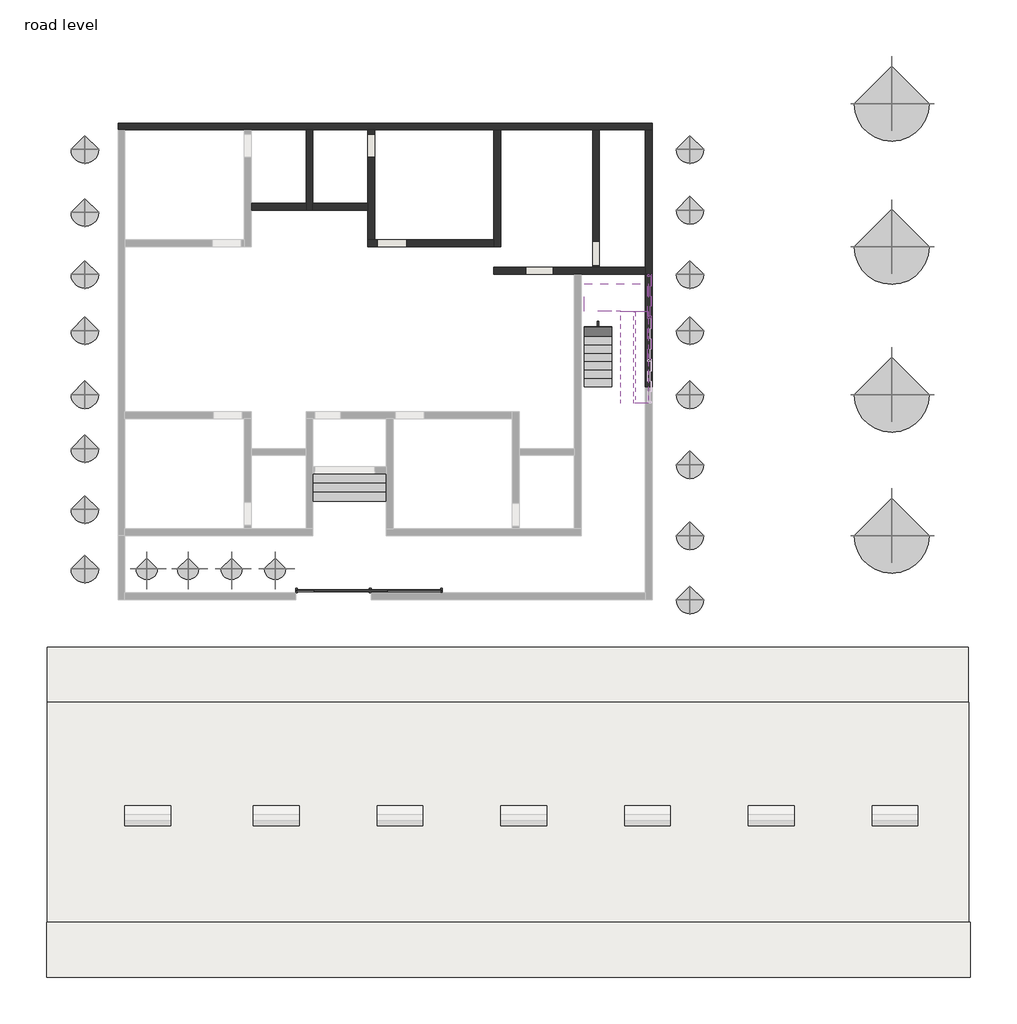
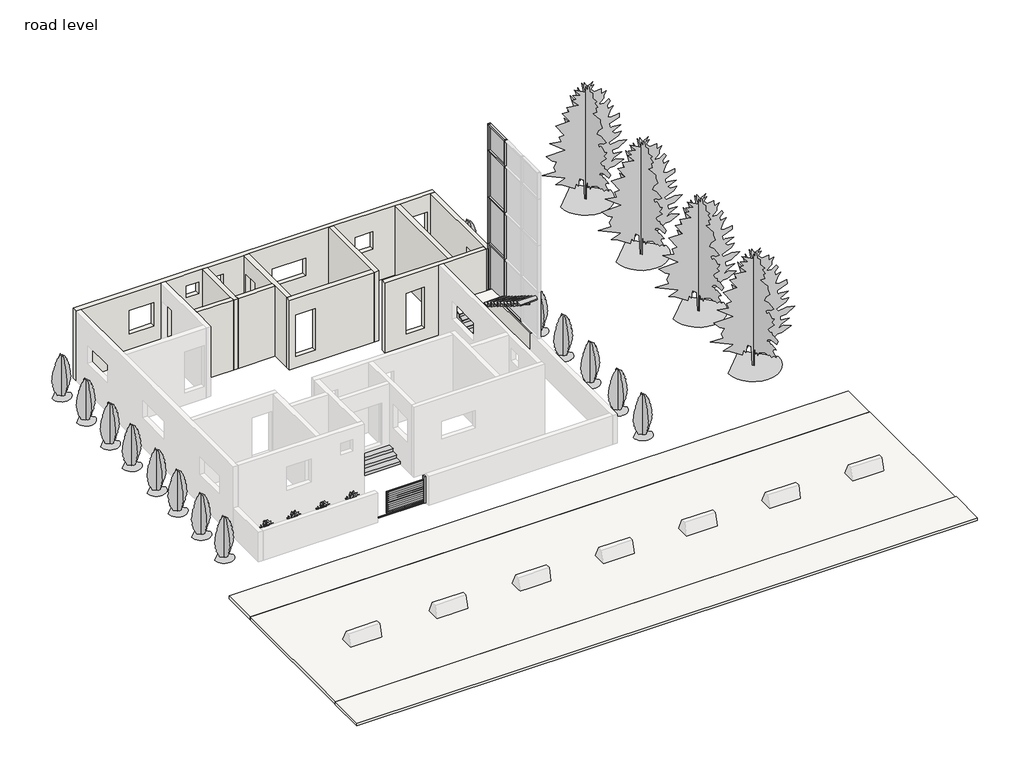
# One storey, part 2 of 2: 25 geographic elements, 16 members, 11 walls, 4 plates, 4 slabs, 2 stair flights, 1 furniture element.
"""IFC4 building model written with IfcOpenShell, lengths in millimetres."""

from ifc_helpers import new_model, si_unit, frame, origin, origin_with_axes, place, context, project, spatial, polyline, outline, extrude, faceted_brep, transform, mapped, element, save
from components import casework_1_casework_1_59e189ff, rpc_plant_tropical_5a024449, rpc_tree_conifer_331a7903, rpc_tree_conifer_chinese_juniper_7_1b9786cd, sliding_gate_17236_sliding_gate_17236_fdb57db6, member_6e705821, member_22948727, member_0bf151aa, member_f0fea5a5, member_ee409385, member_824a4a8d, member_c6627131, system_panel_glazed_532211e4, system_panel_glazed_e2c3efe7, system_panel_glazed_7e5d82eb, non_monolithic_landing_cdb44c8c, stair_flight_ed17b8c2, stair_flight_ca9b9272

model = new_model("IFC4")

# Units and contexts
model_context = context("Model", 3, world=origin())
ifc_project = project(units=[si_unit("LENGTHUNIT", "METRE", prefix="MILLI")], contexts=[model_context])

# Site, building, storey
site = spatial("IfcSite", under=ifc_project)
building = spatial("IfcBuilding", under=site)
storey = spatial("IfcBuildingStorey", under=building, Name="road level", Elevation=0.0)

# Furniture
placement = place(None, origin())
casework_1_casework_1_shape = casework_1_casework_1_59e189ff(model_context)
element("IfcFurniture", 1, ObjectType="Casework 1 : Casework 1", at=placement, inside=storey, context=model_context, shape_type="MappedRepresentation", body=[
    mapped(casework_1_casework_1_shape, transform((0.0, 2082.8, -1435.1), x_axis=(1.0, 0.0, 0.0), y_axis=(0.0, 1.0, 0.0), z_axis=(0.0, 0.0, 1.0))),
])

# Geographic elements
rpc_plant_tropical_shape = rpc_plant_tropical_5a024449(model_context)
element("IfcGeographicElement", 2, ObjectType="RPC Plant - Tropical", at=placement, inside=storey, context=model_context, shape_type="MappedRepresentation", body=[
    mapped(rpc_plant_tropical_shape, transform((-7077.0739162, -7746.9339187, 0.0), x_axis=(1.0, 0.0, 0.0), y_axis=(0.0, 1.0, 0.0), z_axis=(0.0, 0.0, 1.0))),
])
element("IfcGeographicElement", 3, ObjectType="RPC Plant - Tropical", at=placement, inside=storey, context=model_context, shape_type="MappedRepresentation", body=[
    mapped(rpc_plant_tropical_shape, transform((-5705.4739162, -7746.9339187, 0.0), x_axis=(1.0, 0.0, 0.0), y_axis=(0.0, 1.0, 0.0), z_axis=(0.0, 0.0, 1.0))),
])
element("IfcGeographicElement", 4, ObjectType="RPC Plant - Tropical", at=placement, inside=storey, context=model_context, shape_type="MappedRepresentation", body=[
    mapped(rpc_plant_tropical_shape, transform((-4257.6739162, -7746.9339187, 0.0), x_axis=(1.0, 0.0, 0.0), y_axis=(0.0, 1.0, 0.0), z_axis=(0.0, 0.0, 1.0))),
])
element("IfcGeographicElement", 5, ObjectType="RPC Plant - Tropical", at=placement, inside=storey, context=model_context, shape_type="MappedRepresentation", body=[
    mapped(rpc_plant_tropical_shape, transform((-2809.8739162, -7746.9339187, 0.0), x_axis=(1.0, 0.0, 0.0), y_axis=(0.0, 1.0, 0.0), z_axis=(0.0, 0.0, 1.0))),
])
rpc_tree_conifer_shape = rpc_tree_conifer_331a7903(model_context)
element("IfcGeographicElement", 6, ObjectType="RPC Tree - Conifer", at=placement, inside=storey, context=model_context, shape_type="MappedRepresentation", body=[
    mapped(rpc_tree_conifer_shape, transform((17687.9927951, 7721.6660813, 0.0), x_axis=(1.0, 0.0, 0.0), y_axis=(0.0, 1.0, 0.0), z_axis=(0.0, 0.0, 1.0))),
])
element("IfcGeographicElement", 7, ObjectType="RPC Tree - Conifer", at=placement, inside=storey, context=model_context, shape_type="MappedRepresentation", body=[
    mapped(rpc_tree_conifer_shape, transform((17687.9927951, 2959.1660813, 0.0), x_axis=(1.0, 0.0, 0.0), y_axis=(0.0, 1.0, 0.0), z_axis=(0.0, 0.0, 1.0))),
])
element("IfcGeographicElement", 8, ObjectType="RPC Tree - Conifer", at=placement, inside=storey, context=model_context, shape_type="MappedRepresentation", body=[
    mapped(rpc_tree_conifer_shape, transform((17687.9927951, -1955.7339187, 0.0), x_axis=(1.0, 0.0, 0.0), y_axis=(0.0, 1.0, 0.0), z_axis=(0.0, 0.0, 1.0))),
])
element("IfcGeographicElement", 9, ObjectType="RPC Tree - Conifer", at=placement, inside=storey, context=model_context, shape_type="MappedRepresentation", body=[
    mapped(rpc_tree_conifer_shape, transform((17687.9927951, -6642.0339187, 0.0), x_axis=(1.0, 0.0, 0.0), y_axis=(0.0, 1.0, 0.0), z_axis=(0.0, 0.0, 1.0))),
])
rpc_tree_conifer_chinese_juniper_7_shape = rpc_tree_conifer_chinese_juniper_7_1b9786cd(model_context)
element("IfcGeographicElement", 10, ObjectType="RPC Tree - Conifer : Chinese Juniper - 7'", at=placement, inside=storey, context=model_context, shape_type="MappedRepresentation", body=[
    mapped(rpc_tree_conifer_chinese_juniper_7_shape, transform((10982.3927951, 6197.6660813, 0.0), x_axis=(1.0, 0.0, 0.0), y_axis=(0.0, 1.0, 0.0), z_axis=(0.0, 0.0, 1.0))),
])
element("IfcGeographicElement", 11, ObjectType="RPC Tree - Conifer : Chinese Juniper - 7'", at=placement, inside=storey, context=model_context, shape_type="MappedRepresentation", body=[
    mapped(rpc_tree_conifer_chinese_juniper_7_shape, transform((10982.3927951, 4178.3660813, 0.0), x_axis=(1.0, 0.0, 0.0), y_axis=(0.0, 1.0, 0.0), z_axis=(0.0, 0.0, 1.0))),
])
element("IfcGeographicElement", 12, ObjectType="RPC Tree - Conifer : Chinese Juniper - 7'", at=placement, inside=storey, context=model_context, shape_type="MappedRepresentation", body=[
    mapped(rpc_tree_conifer_chinese_juniper_7_shape, transform((10982.3927951, 2044.7660813, 0.0), x_axis=(1.0, 0.0, 0.0), y_axis=(0.0, 1.0, 0.0), z_axis=(0.0, 0.0, 1.0))),
])
element("IfcGeographicElement", 13, ObjectType="RPC Tree - Conifer : Chinese Juniper - 7'", at=placement, inside=storey, context=model_context, shape_type="MappedRepresentation", body=[
    mapped(rpc_tree_conifer_chinese_juniper_7_shape, transform((10982.3927951, 177.8660813, 0.0), x_axis=(1.0, 0.0, 0.0), y_axis=(0.0, 1.0, 0.0), z_axis=(0.0, 0.0, 1.0))),
])
element("IfcGeographicElement", 14, ObjectType="RPC Tree - Conifer : Chinese Juniper - 7'", at=placement, inside=storey, context=model_context, shape_type="MappedRepresentation", body=[
    mapped(rpc_tree_conifer_chinese_juniper_7_shape, transform((10982.3927951, -1955.7339187, 0.0), x_axis=(1.0, 0.0, 0.0), y_axis=(0.0, 1.0, 0.0), z_axis=(0.0, 0.0, 1.0))),
])
element("IfcGeographicElement", 15, ObjectType="RPC Tree - Conifer : Chinese Juniper - 7'", at=placement, inside=storey, context=model_context, shape_type="MappedRepresentation", body=[
    mapped(rpc_tree_conifer_chinese_juniper_7_shape, transform((10982.3927951, -4279.8339187, 0.0), x_axis=(1.0, 0.0, 0.0), y_axis=(0.0, 1.0, 0.0), z_axis=(0.0, 0.0, 1.0))),
])
element("IfcGeographicElement", 16, ObjectType="RPC Tree - Conifer : Chinese Juniper - 7'", at=placement, inside=storey, context=model_context, shape_type="MappedRepresentation", body=[
    mapped(rpc_tree_conifer_chinese_juniper_7_shape, transform((10982.3927951, -6642.0339187, 0.0), x_axis=(1.0, 0.0, 0.0), y_axis=(0.0, 1.0, 0.0), z_axis=(0.0, 0.0, 1.0))),
])
element("IfcGeographicElement", 17, ObjectType="RPC Tree - Conifer : Chinese Juniper - 7'", at=placement, inside=storey, context=model_context, shape_type="MappedRepresentation", body=[
    mapped(rpc_tree_conifer_chinese_juniper_7_shape, transform((10982.3927951, -8775.0319901, 0.0), x_axis=(1.0, 0.0, 0.0), y_axis=(0.0, 1.0, 0.0), z_axis=(0.0, 0.0, 1.0))),
])
element("IfcGeographicElement", 18, ObjectType="RPC Tree - Conifer : Chinese Juniper - 7'", at=placement, inside=storey, context=model_context, shape_type="MappedRepresentation", body=[
    mapped(rpc_tree_conifer_chinese_juniper_7_shape, transform((-9134.6705873, 6197.6660813, 0.0), x_axis=(1.0, 0.0, 0.0), y_axis=(0.0, 1.0, 0.0), z_axis=(0.0, 0.0, 1.0))),
])
element("IfcGeographicElement", 19, ObjectType="RPC Tree - Conifer : Chinese Juniper - 7'", at=placement, inside=storey, context=model_context, shape_type="MappedRepresentation", body=[
    mapped(rpc_tree_conifer_chinese_juniper_7_shape, transform((-9134.6705873, 4102.1660813, 0.0), x_axis=(1.0, 0.0, 0.0), y_axis=(0.0, 1.0, 0.0), z_axis=(0.0, 0.0, 1.0))),
])
element("IfcGeographicElement", 20, ObjectType="RPC Tree - Conifer : Chinese Juniper - 7'", at=placement, inside=storey, context=model_context, shape_type="MappedRepresentation", body=[
    mapped(rpc_tree_conifer_chinese_juniper_7_shape, transform((-9134.6705873, 2044.7660813, 0.0), x_axis=(1.0, 0.0, 0.0), y_axis=(0.0, 1.0, 0.0), z_axis=(0.0, 0.0, 1.0))),
])
element("IfcGeographicElement", 21, ObjectType="RPC Tree - Conifer : Chinese Juniper - 7'", at=placement, inside=storey, context=model_context, shape_type="MappedRepresentation", body=[
    mapped(rpc_tree_conifer_chinese_juniper_7_shape, transform((-9134.6705873, 177.8660813, 0.0), x_axis=(1.0, 0.0, 0.0), y_axis=(0.0, 1.0, 0.0), z_axis=(0.0, 0.0, 1.0))),
])
element("IfcGeographicElement", 22, ObjectType="RPC Tree - Conifer : Chinese Juniper - 7'", at=placement, inside=storey, context=model_context, shape_type="MappedRepresentation", body=[
    mapped(rpc_tree_conifer_chinese_juniper_7_shape, transform((-9134.6705873, -1955.7339187, 0.0), x_axis=(1.0, 0.0, 0.0), y_axis=(0.0, 1.0, 0.0), z_axis=(0.0, 0.0, 1.0))),
])
element("IfcGeographicElement", 23, ObjectType="RPC Tree - Conifer : Chinese Juniper - 7'", at=placement, inside=storey, context=model_context, shape_type="MappedRepresentation", body=[
    mapped(rpc_tree_conifer_chinese_juniper_7_shape, transform((-9134.6705873, -3746.4339187, 0.0), x_axis=(1.0, 0.0, 0.0), y_axis=(0.0, 1.0, 0.0), z_axis=(0.0, 0.0, 1.0))),
])
element("IfcGeographicElement", 24, ObjectType="RPC Tree - Conifer : Chinese Juniper - 7'", at=placement, inside=storey, context=model_context, shape_type="MappedRepresentation", body=[
    mapped(rpc_tree_conifer_chinese_juniper_7_shape, transform((-9134.6705873, -5765.7339187, 0.0), x_axis=(1.0, 0.0, 0.0), y_axis=(0.0, 1.0, 0.0), z_axis=(0.0, 0.0, 1.0))),
])
element("IfcGeographicElement", 25, ObjectType="RPC Tree - Conifer : Chinese Juniper - 7'", at=placement, inside=storey, context=model_context, shape_type="MappedRepresentation", body=[
    mapped(rpc_tree_conifer_chinese_juniper_7_shape, transform((-9134.6705873, -7746.9339187, 0.0), x_axis=(1.0, 0.0, 0.0), y_axis=(0.0, 1.0, 0.0), z_axis=(0.0, 0.0, 1.0))),
])
sliding_gate_17236_sliding_gate_17236_shape = sliding_gate_17236_sliding_gate_17236_fdb57db6(model_context)
element("IfcGeographicElement", 26, ObjectType="Sliding_Gate_17236 : Sliding_Gate_17236", at=placement, inside=storey, context=model_context, shape_type="MappedRepresentation", body=[
    mapped(sliding_gate_17236_sliding_gate_17236_shape, transform((-2124.0739162, -8546.4319901, 0.0), x_axis=(1.0, 0.0, 0.0), y_axis=(0.0, 1.0, 0.0), z_axis=(0.0, 0.0, 1.0))),
])

# Members
element("IfcMember", 27, ObjectType="Carriage - 2\" Width", at=placement, inside=storey, context=model_context, shape_type="SweptSolid", body=[
    extrude(outline(polyline([(825.5660813, 1507.8363636), (825.5660813, 1413.447706), (-1454.7962178, 0.0), (-1657.2839187, 0.0), (-1657.2839187, 122.3818182), (-1377.8839187, 122.3818182), (-1377.8839187, 295.5636364), (-1098.4839187, 295.5636364), (-1098.4839187, 468.7454545), (-819.0839187, 468.7454545), (-819.0839187, 641.9272727), (-539.6839187, 641.9272727), (-539.6839187, 815.1090909), (-260.2839187, 815.1090909), (-260.2839187, 988.2909091), (19.1160813, 988.2909091), (19.1160813, 1161.4727273), (298.5160813, 1161.4727273), (298.5160813, 1334.6545455), (577.9160813, 1334.6545455), (577.9160813, 1507.8363636), (825.5660813, 1507.8363636)])), frame((7896.2260838, 0.0, 0.0), z_axis=(1.0, 0.0, 0.0), x_axis=(0.0, 1.0, 0.0)), (0.0, 0.0, 1.0), 50.8),
])
element("IfcMember", 28, ObjectType="Carriage - 2\" Width", at=placement, inside=storey, context=model_context, shape_type="SweptSolid", body=[
    extrude(outline(polyline([(-2247.8339187, 3491.6295242), (-2247.8339187, 3586.0181818), (-2000.1839187, 3586.0181818), (-2000.1839187, 3412.8363636), (-1720.7839187, 3412.8363636), (-1720.7839187, 3239.6545455), (-1441.3839187, 3239.6545455), (-1441.3839187, 3066.4727273), (-1161.9839187, 3066.4727273), (-1161.9839187, 2893.2909091), (-882.5839187, 2893.2909091), (-882.5839187, 2720.1090909), (-603.1839187, 2720.1090909), (-603.1839187, 2546.9272727), (-323.7839187, 2546.9272727), (-323.7839187, 2373.7454545), (-44.3839187, 2373.7454545), (-44.3839187, 2200.5636364), (235.0160813, 2200.5636364), (235.0160813, 2027.3818182), (514.4160813, 2027.3818182), (514.4160813, 1854.2), (793.8160813, 1854.2), (793.8160813, 1606.3092763), (-2247.8339187, 3491.6295242)])), frame((9115.4260838, 0.0, 0.0), z_axis=(1.0, 0.0, 0.0), x_axis=(0.0, 1.0, 0.0)), (0.0, 0.0, 1.0), 50.8),
])
member_shape = member_6e705821(model_context)
element("IfcMember", 29, ObjectType="Rectangular Mullion : 2.5\" x 5\" rectangular", at=placement, inside=storey, context=model_context, shape_type="MappedRepresentation", body=[
    mapped(member_shape, transform((9636.3894662, 645.6494146, 10210.8), x_axis=(0.0, 0.0, 1.0), y_axis=(-1.0, 0.0, 0.0), z_axis=(0.0, -1.0, 0.0))),
])
element("IfcMember", 30, ObjectType="Rectangular Mullion : 2.5\" x 5\" rectangular", at=placement, inside=storey, context=model_context, shape_type="MappedRepresentation", body=[
    mapped(member_shape, transform((9636.3894662, 1981.2660813, 1524.0), x_axis=(0.0, 0.0, -1.0), y_axis=(-1.0, 0.0, 0.0), z_axis=(0.0, 1.0, 0.0))),
])
member_2_shape = member_22948727(model_context)
element("IfcMember", 31, ObjectType="Rectangular Mullion : 2.5\" x 5\" rectangular", at=placement, inside=storey, context=model_context, shape_type="MappedRepresentation", body=[
    mapped(member_2_shape, transform((9636.3894662, 582.1494146, 1524.0), x_axis=(0.0, 0.0, -1.0), y_axis=(-1.0, 0.0, 0.0), z_axis=(0.0, 1.0, 0.0))),
])
member_3_shape = member_0bf151aa(model_context)
element("IfcMember", 32, ObjectType="Rectangular Mullion : 2.5\" x 5\" rectangular", at=placement, inside=storey, context=model_context, shape_type="MappedRepresentation", body=[
    mapped(member_3_shape, transform((9636.3894662, 645.6494146, 3962.4), x_axis=(0.0, 0.0, 1.0), y_axis=(-1.0, 0.0, 0.0), z_axis=(0.0, -1.0, 0.0))),
])
element("IfcMember", 33, ObjectType="Rectangular Mullion : 2.5\" x 5\" rectangular", at=placement, inside=storey, context=model_context, shape_type="MappedRepresentation", body=[
    mapped(member_3_shape, transform((9636.3894662, 645.6494146, 6400.8), x_axis=(0.0, 0.0, 1.0), y_axis=(-1.0, 0.0, 0.0), z_axis=(0.0, -1.0, 0.0))),
])
element("IfcMember", 34, ObjectType="Rectangular Mullion : 2.5\" x 5\" rectangular", at=placement, inside=storey, context=model_context, shape_type="MappedRepresentation", body=[
    mapped(member_3_shape, transform((9636.3894662, 645.6494146, 8839.2), x_axis=(0.0, 0.0, 1.0), y_axis=(-1.0, 0.0, 0.0), z_axis=(0.0, -1.0, 0.0))),
])
member_4_shape = member_f0fea5a5(model_context)
element("IfcMember", 35, ObjectType="Rectangular Mullion : 2.5\" x 5\" rectangular", at=placement, inside=storey, context=model_context, shape_type="MappedRepresentation", body=[
    mapped(member_4_shape, transform((9636.3894662, 613.8994146, 1524.0), x_axis=(0.0, -1.0, 0.0), y_axis=(-1.0, 0.0, 0.0), z_axis=(0.0, 0.0, -1.0))),
])
element("IfcMember", 36, ObjectType="Rectangular Mullion : 2.5\" x 5\" rectangular", at=placement, inside=storey, context=model_context, shape_type="MappedRepresentation", body=[
    mapped(member_4_shape, transform((9636.3894662, 613.8994146, 3962.4), x_axis=(0.0, -1.0, 0.0), y_axis=(-1.0, 0.0, 0.0), z_axis=(0.0, 0.0, -1.0))),
])
element("IfcMember", 37, ObjectType="Rectangular Mullion : 2.5\" x 5\" rectangular", at=placement, inside=storey, context=model_context, shape_type="MappedRepresentation", body=[
    mapped(member_4_shape, transform((9636.3894662, 613.8994146, 6400.8), x_axis=(0.0, -1.0, 0.0), y_axis=(-1.0, 0.0, 0.0), z_axis=(0.0, 0.0, -1.0))),
])
member_5_shape = member_ee409385(model_context)
element("IfcMember", 38, ObjectType="Rectangular Mullion : 2.5\" x 5\" rectangular", at=placement, inside=storey, context=model_context, shape_type="MappedRepresentation", body=[
    mapped(member_5_shape, transform((9636.3894662, 2044.7660813, 3962.4), x_axis=(0.0, 1.0, 0.0), y_axis=(-1.0, 0.0, 0.0), z_axis=(0.0, 0.0, 1.0))),
])
element("IfcMember", 39, ObjectType="Rectangular Mullion : 2.5\" x 5\" rectangular", at=placement, inside=storey, context=model_context, shape_type="MappedRepresentation", body=[
    mapped(member_5_shape, transform((9636.3894662, 2044.7660813, 6400.8), x_axis=(0.0, 1.0, 0.0), y_axis=(-1.0, 0.0, 0.0), z_axis=(0.0, 0.0, 1.0))),
])
element("IfcMember", 40, ObjectType="Rectangular Mullion : 2.5\" x 5\" rectangular", at=placement, inside=storey, context=model_context, shape_type="MappedRepresentation", body=[
    mapped(member_5_shape, transform((9636.3894662, 2044.7660813, 8839.2), x_axis=(0.0, 1.0, 0.0), y_axis=(-1.0, 0.0, 0.0), z_axis=(0.0, 0.0, 1.0))),
])
member_6_shape = member_824a4a8d(model_context)
element("IfcMember", 41, ObjectType="Rectangular Mullion : 2.5\" x 5\" rectangular", at=placement, inside=storey, context=model_context, shape_type="MappedRepresentation", body=[
    mapped(member_6_shape, transform((9636.3894662, 613.8994146, 8839.2), x_axis=(0.0, -1.0, 0.0), y_axis=(-1.0, 0.0, 0.0), z_axis=(0.0, 0.0, -1.0))),
])
member_7_shape = member_c6627131(model_context)
element("IfcMember", 42, ObjectType="Rectangular Mullion : 2.5\" x 5\" rectangular", at=placement, inside=storey, context=model_context, shape_type="MappedRepresentation", body=[
    mapped(member_7_shape, transform((9636.3894662, 2044.7660813, 10210.8), x_axis=(0.0, 1.0, 0.0), y_axis=(-1.0, 0.0, 0.0), z_axis=(0.0, 0.0, 1.0))),
])

# Plates
system_panel_glazed_shape = system_panel_glazed_532211e4(model_context)
element("IfcPlate", 43, ObjectType="System Panel : Glazed", at=placement, inside=storey, context=model_context, shape_type="MappedRepresentation", body=[
    mapped(system_panel_glazed_shape, transform((9636.3894662, 1313.4577479, 1587.5), x_axis=(0.0, -1.0, 0.0), y_axis=(1.0, 0.0, 0.0), z_axis=(0.0, 0.0, 1.0))),
])
system_panel_glazed_2_shape = system_panel_glazed_e2c3efe7(model_context)
element("IfcPlate", 44, ObjectType="System Panel : Glazed", at=placement, inside=storey, context=model_context, shape_type="MappedRepresentation", body=[
    mapped(system_panel_glazed_2_shape, transform((9636.3894662, 1313.4577479, 3994.15), x_axis=(0.0, -1.0, 0.0), y_axis=(1.0, 0.0, 0.0), z_axis=(0.0, 0.0, 1.0))),
])
element("IfcPlate", 45, ObjectType="System Panel : Glazed", at=placement, inside=storey, context=model_context, shape_type="MappedRepresentation", body=[
    mapped(system_panel_glazed_2_shape, transform((9636.3894662, 1313.4577479, 6432.55), x_axis=(0.0, -1.0, 0.0), y_axis=(1.0, 0.0, 0.0), z_axis=(0.0, 0.0, 1.0))),
])
system_panel_glazed_3_shape = system_panel_glazed_7e5d82eb(model_context)
element("IfcPlate", 46, ObjectType="System Panel : Glazed", at=placement, inside=storey, context=model_context, shape_type="MappedRepresentation", body=[
    mapped(system_panel_glazed_3_shape, transform((9636.3894662, 1313.4577479, 8870.95), x_axis=(0.0, -1.0, 0.0), y_axis=(1.0, 0.0, 0.0), z_axis=(0.0, 0.0, 1.0))),
])

# Slabs
element("IfcSlab", 47, ObjectType="Generic - 6\"", at=placement, inside=storey, context=model_context, shape_type="SweptSolid", body=[
    extrude(outline(polyline([(20239.3163133, -10350.487401), (20239.3163133, -12179.287401), (-10393.0836867, -12179.287401), (-10393.0836867, -10350.487401), (20239.3163133, -10350.487401)])), frame((0.0, 0.0, -152.4), z_axis=(0.0, 0.0, 1.0), x_axis=(1.0, 0.0, 0.0)), (0.0, 0.0, 1.0), 152.4),
])
element("IfcSlab", 48, ObjectType="Generic - 6\"", at=placement, inside=storey, context=model_context, shape_type="SweptSolid", body=[
    extrude(outline(polyline([(20300.1913625, -19501.3971684), (20300.1913625, -21330.1971684), (-10408.4086375, -21330.1971684), (-10408.4086375, -19501.3971684), (20300.1913625, -19501.3971684)])), frame((0.0, 0.0, -152.4), z_axis=(0.0, 0.0, 1.0), x_axis=(1.0, 0.0, 0.0)), (0.0, 0.0, 1.0), 152.4),
])
element("IfcSlab", 49, ObjectType="Generic - 6\" 3", at=placement, inside=storey, context=model_context, shape_type="SweptSolid", body=[
    extrude(outline(polyline([(20253.6498617, -12186.0365182), (20253.6498617, -19501.2365182), (-10391.4501383, -19501.2365182), (-10391.4501383, -12186.0365182), (20253.6498617, -12186.0365182)])), frame((0.0, 0.0, -152.4), z_axis=(0.0, 0.0, 1.0), x_axis=(1.0, 0.0, 0.0)), (0.0, 0.0, 1.0), 152.4),
])
non_monolithic_landing_shape = non_monolithic_landing_cdb44c8c(model_context)
element("IfcSlab", 50, ObjectType="Non-Monolithic Landing", at=placement, inside=storey, context=model_context, shape_type="MappedRepresentation", body=[
    mapped(non_monolithic_landing_shape, transform((0.0, 0.0, 0.0), x_axis=(1.0, 0.0, 0.0), y_axis=(0.0, 1.0, 0.0), z_axis=(0.0, 0.0, 1.0))),
])

# Stair flights
stair_flight_shape = stair_flight_ed17b8c2(model_context)
element("IfcStairFlight", 51, ObjectType="2\" Tread 1\" Nosing 1/4\" Riser", at=placement, inside=storey, context=model_context, shape_type="MappedRepresentation", body=[
    mapped(stair_flight_shape, transform((0.0, 0.0, 0.0), x_axis=(1.0, 0.0, 0.0), y_axis=(0.0, 1.0, 0.0), z_axis=(0.0, 0.0, 1.0))),
])
stair_flight_2_shape = stair_flight_ca9b9272(model_context)
element("IfcStairFlight", 52, ObjectType="2\" Tread 1\" Nosing 1/4\" Riser", at=placement, inside=storey, context=model_context, shape_type="MappedRepresentation", body=[
    mapped(stair_flight_2_shape, transform((0.0, 0.0, 0.0), x_axis=(1.0, 0.0, 0.0), y_axis=(0.0, 1.0, 0.0), z_axis=(0.0, 0.0, 1.0))),
])

# Walls
element("IfcWall", 53, ObjectType="Generic - 9\"", at=placement, inside=storey, context=model_context, shape_type="Brep", body=[
    faceted_brep([(-8029.5739162, 6845.3660813, 0.0), (-7800.9739162, 6845.3660813, 0.0), (-3838.5739162, 6845.3660813, 0.0), (-3609.9739162, 6845.3660813, 0.0), (-1781.1739162, 6845.3660813, 0.0), (-1552.5739162, 6845.3660813, 0.0), (276.2260838, 6845.3660813, 0.0), (504.8260838, 6845.3660813, 0.0), (4467.2260838, 6845.3660813, 0.0), (4695.8260838, 6845.3660813, 0.0), (7743.8260838, 6845.3660813, 0.0), (7972.4260838, 6845.3660813, 0.0), (9496.6894662, 6845.3660813, 0.0), (9725.2894662, 6845.3660813, 0.0), (9725.2894662, 6845.3660813, 3657.6), (9496.6894662, 6845.3660813, 3657.6), (7972.4260838, 6845.3660813, 3657.6), (7743.8260838, 6845.3660813, 3657.6), (4695.8260838, 6845.3660813, 3657.6), (4467.2260838, 6845.3660813, 3657.6), (504.8260838, 6845.3660813, 3657.6), (276.2260838, 6845.3660813, 3657.6), (-1552.5739162, 6845.3660813, 3657.6), (-1781.1739162, 6845.3660813, 3657.6), (-3609.9739162, 6845.3660813, 3657.6), (-3838.5739162, 6845.3660813, 3657.6), (-7800.9739162, 6845.3660813, 3657.6), (-8029.5739162, 6845.3660813, 3657.6), (3324.2260838, 6845.3660813, 2438.4), (3324.2260838, 6845.3660813, 1524.0), (1673.2260838, 6845.3660813, 1524.0), (1673.2260838, 6845.3660813, 2438.4), (9344.0260838, 6845.3660813, 2743.2), (9344.0260838, 6845.3660813, 1524.0), (8124.8260838, 6845.3660813, 1524.0), (8124.8260838, 6845.3660813, 2743.2), (-2581.2739162, 6845.3660813, 3048.0), (-1971.6739162, 6845.3660813, 3048.0), (-1971.6739162, 6845.3660813, 2438.4), (-2581.2739162, 6845.3660813, 2438.4), (-1362.0739162, 6845.3660813, 3048.0), (-752.4739162, 6845.3660813, 3048.0), (-752.4739162, 6845.3660813, 2438.4), (-1362.0739162, 6845.3660813, 2438.4), (-4181.4739162, 6845.3660813, 2743.2), (-4181.4739162, 6845.3660813, 1524.0), (-5400.6739162, 6845.3660813, 1524.0), (-5400.6739162, 6845.3660813, 2743.2), (6651.6260838, 6845.3660813, 2667.0), (6651.6260838, 6845.3660813, 1752.6), (5788.0260838, 6845.3660813, 1752.6), (5788.0260838, 6845.3660813, 2667.0), (-8029.5739162, 7073.9660813, 0.0), (-8029.5739162, 7073.9660813, 3657.6), (9725.2894662, 7073.9660813, 3657.6), (9725.2894662, 7073.9660813, 0.0), (3324.2260838, 7073.9660813, 2438.4), (1673.2260838, 7073.9660813, 2438.4), (1673.2260838, 7073.9660813, 1524.0), (3324.2260838, 7073.9660813, 1524.0), (9344.0260838, 7073.9660813, 2743.2), (8124.8260838, 7073.9660813, 2743.2), (8124.8260838, 7073.9660813, 1524.0), (9344.0260838, 7073.9660813, 1524.0), (-2581.2739162, 7073.9660813, 3048.0), (-2581.2739162, 7073.9660813, 2438.4), (-1971.6739162, 7073.9660813, 2438.4), (-1971.6739162, 7073.9660813, 3048.0), (-1362.0739162, 7073.9660813, 3048.0), (-1362.0739162, 7073.9660813, 2438.4), (-752.4739162, 7073.9660813, 2438.4), (-752.4739162, 7073.9660813, 3048.0), (-4181.4739162, 7073.9660813, 2743.2), (-5400.6739162, 7073.9660813, 2743.2), (-5400.6739162, 7073.9660813, 1524.0), (-4181.4739162, 7073.9660813, 1524.0), (6651.6260838, 7073.9660813, 2667.0), (5788.0260838, 7073.9660813, 2667.0), (5788.0260838, 7073.9660813, 1752.6), (6651.6260838, 7073.9660813, 1752.6)], [[[0, 1, 2, 3, 4, 5, 6, 7, 8, 9, 10, 11, 12, 13, 14, 15, 16, 17, 18, 19, 20, 21, 22, 23, 24, 25, 26, 27], [28, 29, 30, 31], [32, 33, 34, 35], [36, 37, 38, 39], [40, 41, 42, 43], [44, 45, 46, 47], [48, 49, 50, 51]], [[52, 53, 54, 55], [56, 57, 58, 59], [60, 61, 62, 63], [64, 65, 66, 67], [68, 69, 70, 71], [72, 73, 74, 75], [76, 77, 78, 79]], [[13, 12, 11, 10, 9, 8, 7, 6, 5, 4, 3, 2, 1, 0, 52, 55]], [[0, 27, 53, 52]], [[14, 13, 55, 54]], [[29, 28, 56, 59]], [[30, 29, 59, 58]], [[31, 30, 58, 57]], [[28, 31, 57, 56]], [[33, 32, 60, 63]], [[34, 33, 63, 62]], [[35, 34, 62, 61]], [[32, 35, 61, 60]], [[65, 64, 36, 39]], [[66, 65, 39, 38]], [[67, 66, 38, 37]], [[64, 67, 37, 36]], [[69, 68, 40, 43]], [[70, 69, 43, 42]], [[71, 70, 42, 41]], [[68, 71, 41, 40]], [[45, 44, 72, 75]], [[46, 45, 75, 74]], [[47, 46, 74, 73]], [[44, 47, 73, 72]], [[49, 48, 76, 79]], [[50, 49, 79, 78]], [[51, 50, 78, 77]], [[48, 51, 77, 76]], [[27, 26, 25, 24, 23, 22, 21, 20, 19, 18, 17, 16, 15, 14, 54, 53]]]),
])
element("IfcWall", 54, ObjectType="Generic - 9\"", at=placement, inside=storey, context=model_context, shape_type="Brep", body=[
    faceted_brep([(-1781.1739162, 6845.3660813, 0.0), (-1781.1739162, 4406.9660813, 0.0), (-1781.1739162, 4178.3660813, 0.0), (-1781.1739162, 4178.3660813, 3657.6), (-1781.1739162, 4406.9660813, 3657.6), (-1781.1739162, 6845.3660813, 3657.6), (-1552.5739162, 6845.3660813, 0.0), (-1552.5739162, 6845.3660813, 3657.6), (-1552.5739162, 4406.9660813, 3657.6), (-1552.5739162, 4178.3660813, 3657.6), (-1552.5739162, 4178.3660813, 0.0), (-1552.5739162, 4406.9660813, 0.0)], [[[0, 1, 2, 3, 4, 5]], [[6, 7, 8, 9, 10, 11]], [[2, 1, 0, 6, 11, 10]], [[0, 5, 7, 6]], [[3, 2, 10, 9]], [[5, 4, 3, 9, 8, 7]]]),
])
element("IfcWall", 55, ObjectType="Generic - 9\"", at=placement, inside=storey, context=model_context, shape_type="Brep", body=[
    faceted_brep([(276.2260838, 6845.3660813, 0.0), (276.2260838, 4406.9660813, 0.0), (276.2260838, 4178.3660813, 0.0), (276.2260838, 3187.7660813, 0.0), (276.2260838, 3187.7660813, 3657.6), (276.2260838, 4178.3660813, 3657.6), (276.2260838, 4406.9660813, 3657.6), (276.2260838, 6845.3660813, 3657.6), (276.2260838, 5943.6660813, 609.6), (276.2260838, 6705.6660813, 609.6), (276.2260838, 6705.6660813, 2743.2), (276.2260838, 5943.6660813, 2743.2), (504.8260838, 3187.7660813, 0.0), (504.8260838, 6845.3660813, 0.0), (504.8260838, 6845.3660813, 3657.6), (504.8260838, 3187.7660813, 3657.6), (504.8260838, 6705.6660813, 609.6), (504.8260838, 5943.6660813, 609.6), (504.8260838, 5943.6660813, 2743.2), (504.8260838, 6705.6660813, 2743.2)], [[[0, 1, 2, 3, 4, 5, 6, 7], [8, 9, 10, 11]], [[12, 13, 14, 15], [16, 17, 18, 19]], [[3, 2, 1, 0, 13, 12]], [[0, 7, 14, 13]], [[4, 3, 12, 15]], [[8, 17, 16, 9]], [[9, 16, 19, 10]], [[17, 8, 11, 18]], [[18, 11, 10, 19]], [[7, 6, 5, 4, 15, 14]]]),
])
element("IfcWall", 56, ObjectType="Generic - 9\"", at=placement, inside=storey, context=model_context, shape_type="Brep", body=[
    faceted_brep([(4467.2260838, 6845.3660813, 0.0), (4467.2260838, 3187.7660813, 0.0), (4467.2260838, 2959.1660813, 0.0), (4467.2260838, 2959.1660813, 609.6), (4467.2260838, 2959.1660813, 3657.6), (4467.2260838, 3187.7660813, 3657.6), (4467.2260838, 6845.3660813, 3657.6), (4695.8260838, 6845.3660813, 0.0), (4695.8260838, 6845.3660813, 3657.6), (4695.8260838, 2959.1660813, 3657.6), (4695.8260838, 2959.1660813, 609.6), (4695.8260838, 2959.1660813, 0.0)], [[[0, 1, 2, 3, 4, 5, 6]], [[7, 8, 9, 10, 11]], [[2, 1, 0, 7, 11]], [[0, 6, 8, 7]], [[2, 11, 10, 9, 4, 3]], [[6, 5, 4, 9, 8]]]),
])
element("IfcWall", 57, ObjectType="Generic - 9\"", at=placement, inside=storey, context=model_context, shape_type="SweptSolid", body=[
    extrude(outline(polyline([(-3609.9739162, 4406.9660813), (-1781.1739162, 4406.9660813), (-1781.1739162, 4178.3660813), (-3609.9739162, 4178.3660813), (-3609.9739162, 4406.9660813)])), origin_with_axes(), (0.0, 0.0, 1.0), 3657.6),
])
element("IfcWall", 58, ObjectType="Generic - 9\"", at=placement, inside=storey, context=model_context, shape_type="SweptSolid", body=[
    extrude(outline(polyline([(276.2260838, 4178.3660813), (-1552.5739162, 4178.3660813), (-1552.5739162, 4406.9660813), (276.2260838, 4406.9660813), (276.2260838, 4178.3660813)])), origin_with_axes(), (0.0, 0.0, 1.0), 3657.6),
])
element("IfcWall", 59, ObjectType="Generic - 9\"", at=placement, inside=storey, context=model_context, shape_type="Brep", body=[
    faceted_brep([(276.2260838, 2959.1660813, 0.0), (4467.2260838, 2959.1660813, 0.0), (4467.2260838, 2959.1660813, 3657.6), (276.2260838, 2959.1660813, 3657.6), (593.7260838, 2959.1660813, 609.6), (593.7260838, 2959.1660813, 2768.6), (1558.9260838, 2959.1660813, 2768.6), (1558.9260838, 2959.1660813, 609.6), (4467.2260838, 3187.7660813, 0.0), (504.8260838, 3187.7660813, 0.0), (276.2260838, 3187.7660813, 0.0), (276.2260838, 3187.7660813, 3657.6), (504.8260838, 3187.7660813, 3657.6), (4467.2260838, 3187.7660813, 3657.6), (593.7260838, 3187.7660813, 2768.6), (593.7260838, 3187.7660813, 609.6), (1558.9260838, 3187.7660813, 609.6), (1558.9260838, 3187.7660813, 2768.6)], [[[0, 1, 2, 3], [4, 5, 6, 7]], [[8, 9, 10, 11, 12, 13], [14, 15, 16, 17]], [[1, 0, 10, 9, 8]], [[0, 3, 11, 10]], [[4, 15, 14, 5]], [[5, 14, 17, 6]], [[6, 17, 16, 7]], [[15, 4, 7, 16]], [[1, 8, 13, 2]], [[3, 2, 13, 12, 11]]]),
])
element("IfcWall", 60, ObjectType="Generic - 9\"", at=placement, inside=storey, context=model_context, shape_type="SweptSolid", body=[
    extrude(outline(polyline([(6845.3660813, 0.0), (2273.3660813, 0.0), (2273.3660813, 3657.6), (6845.3660813, 3657.6), (6845.3660813, 0.0)]), holes=[polyline([(2336.8660813, 2768.6), (2336.8660813, 609.6), (3149.6660813, 609.6), (3149.6660813, 2768.6), (2336.8660813, 2768.6)])]), frame((7743.8260838, 0.0, 0.0), z_axis=(1.0, 0.0, 0.0), x_axis=(0.0, 1.0, 0.0)), (0.0, 0.0, 1.0), 228.6),
])
element("IfcWall", 61, ObjectType="Generic - 9\"", at=placement, inside=storey, context=model_context, shape_type="Brep", body=[
    faceted_brep([(9496.6894662, 2273.3660813, 0.0), (7972.4260838, 2273.3660813, 0.0), (7743.8260838, 2273.3660813, 0.0), (4467.2260838, 2273.3660813, 0.0), (4467.2260838, 2273.3660813, 609.6), (4467.2260838, 2273.3660813, 3657.6), (4695.8260838, 2273.3660813, 3657.6), (7743.8260838, 2273.3660813, 3657.6), (7972.4260838, 2273.3660813, 3657.6), (9496.6894662, 2273.3660813, 3657.6), (6435.7260838, 2273.3660813, 609.6), (6435.7260838, 2273.3660813, 2743.2), (5521.3260838, 2273.3660813, 2743.2), (5521.3260838, 2273.3660813, 609.6), (4467.2260838, 2044.7660813, 0.0), (7134.2260838, 2044.7660813, 0.0), (7362.8260838, 2044.7660813, 0.0), (9496.6894662, 2044.7660813, 0.0), (9496.6894662, 2044.7660813, 3657.6), (7362.8260838, 2044.7660813, 3657.6), (7134.2260838, 2044.7660813, 3657.6), (4467.2260838, 2044.7660813, 3657.6), (6435.7260838, 2044.7660813, 2743.2), (6435.7260838, 2044.7660813, 609.6), (5521.3260838, 2044.7660813, 609.6), (5521.3260838, 2044.7660813, 2743.2)], [[[0, 1, 2, 3, 4, 5, 6, 7, 8, 9], [10, 11, 12, 13]], [[14, 15, 16, 17, 18, 19, 20, 21], [22, 23, 24, 25]], [[3, 2, 1, 0, 17, 16, 15, 14]], [[5, 4, 3, 14, 21]], [[22, 11, 10, 23]], [[23, 10, 13, 24]], [[24, 13, 12, 25]], [[11, 22, 25, 12]], [[9, 8, 7, 6, 5, 21, 20, 19, 18]], [[17, 0, 9, 18]]]),
])
element("IfcWall", 62, ObjectType="Generic - 9\"", at=placement, inside=storey, context=model_context, shape_type="Brep", body=[
    faceted_brep([(9496.6894662, 6845.3660813, 0.0), (9496.6894662, 2273.3660813, 0.0), (9496.6894662, 2044.7660813, 0.0), (9496.6894662, 2044.7660813, 1524.0), (9496.6894662, 2044.7660813, 3657.6), (9496.6894662, 2273.3660813, 3657.6), (9496.6894662, 6845.3660813, 3657.6), (9496.6894662, 2507.1811041, 2743.2), (9496.6894662, 2507.1811041, 1524.0), (9496.6894662, 3726.3811041, 1524.0), (9496.6894662, 3726.3811041, 2743.2), (9725.2894662, 2044.7660813, 0.0), (9725.2894662, 6845.3660813, 0.0), (9725.2894662, 6845.3660813, 3657.6), (9725.2894662, 2044.7660813, 3657.6), (9725.2894662, 2044.7660813, 1524.0), (9725.2894662, 2507.1811041, 1524.0), (9725.2894662, 2507.1811041, 2743.2), (9725.2894662, 3726.3811041, 2743.2), (9725.2894662, 3726.3811041, 1524.0)], [[[0, 1, 2, 3, 4, 5, 6], [7, 8, 9, 10]], [[11, 12, 13, 14, 15], [16, 17, 18, 19]], [[2, 1, 0, 12, 11]], [[0, 6, 13, 12]], [[7, 17, 16, 8]], [[8, 16, 19, 9]], [[9, 19, 18, 10]], [[17, 7, 10, 18]], [[6, 5, 4, 14, 13]], [[2, 11, 15, 14, 4, 3]]]),
])
element("IfcWall", 63, ObjectType="Generic - 9\"", at=placement, inside=storey, context=model_context, shape_type="Brep", body=[
    faceted_brep([(9496.6894662, 2044.7660813, 0.0), (9496.6894662, -1714.4339187, 0.0), (9496.6894662, -1714.4339187, 1524.0), (9496.6894662, 2044.7660813, 1524.0), (9725.2894662, 2044.7660813, 0.0), (9725.2894662, 2044.7660813, 1524.0), (9725.2894662, -1714.4339187, 1524.0), (9725.2894662, -1714.4339187, 0.0), (9725.0260838, -1714.4339187, 0.0), (9725.0260838, -1714.4339187, 1524.0)], [[[0, 1, 2, 3]], [[4, 5, 6, 7]], [[1, 0, 4, 7, 8]], [[2, 1, 8, 7, 6, 9]], [[3, 2, 9, 6, 5]], [[0, 3, 5, 4]]]),
])

save(model, "model.ifc")

# Revit data of these elements
# Type "RPC Plant - Tropical"
#   built-in parameter 1005198 = "{2, 15},{39, RPC-16-FWM5-GM7X-C67P-4000-ST1L-LVER-AU},{1, 0},{1, 0},{2, 35},{1, 8},{5, Color},{1, 0},{1, 0},{3, 0.8},{3, 0.8},{3, 0.8},{1, 8},{7, BBoxMin},{1, 0},{1, 0},{1, 0},{1, 0},{1, 0},{1, 8},{7, BBoxMax},{1, 0},{1, 0},{1, 0},{1, 0},{1, 0},{2, 11},{9, RPCTypeId},{1, 0},{1, 0},{39, RPC-16-FWM5-GM7X-C67P-4000-ST1L-LVER-AU},{1, 6},{14, RPCPlantHeight},{1, 0},{1, 0},{1, 3},{2, 11},{7, keyword},{1, 0},{1, 0},{99, :Geometry:RPC:Crane Lily:strelitzia:reinae:crane lily:plants:shrub:flower:tropical:bird-of-paradise},{2, 11},{8, category},{1, 0},{1, 0},{17, :Shrubs [General]},{2, 11},{12, LocalizedUID},{1, 0},{1, 0},{10, Crane Lily},{2, 14},{6, Height},{1, 0},{1, 0},{1, 3},{1, 2},{16, Cast Reflections},{1, 0},{1, 0},{1, 0},{1, 2},{12, Cast Shadows},{1, 0},{1, 0},{1, 1},{1, 2},{9, Lock View},{1, 0},{1, 0},{1, 0},{1, 4},{5, ViewC},{1, 0},{1, 0},{1, 0},{2, 11},{20, AdvancedUIDefinition},{1, 0},{1, 0},{0, },{2, 11},{10, AssetLibID},{1, 0},{1, 0},{36, 4D3F6E72-3F99-4203-98E9-AF80B3C7A7A4},{2, 11},{10, BaseSchema},{1, 0},{1, 0},{9, RPCSchema},{2, 11},{12, ExchangeGUID},{1, 0},{1, 0},{0, },{1, 2},{6, Hidden},{1, 0},{1, 0},{1, 0},{1, 4},{11, RPCCategory},{1, 0},{1, 0},{1, 0},{2, 11},{8, RPCImage},{1, 0},{1, 0},{0, },{1, 4},{13, SchemaVersion},{1, 0},{1, 0},{1, 4},{2, 11},{12, UIDefinition},{1, 0},{1, 0},{0, },{2, 11},{6, UIName},{1, 0},{1, 0},{39, RPC-16-FWM5-GM7X-C67P-4000-ST1L-LVER-AU},{2, 11},{11, VersionGUID},{1, 0},{1, 0},{9, RPCSchema},{2, 11},{9, assettype},{1, 0},{1, 0},{11, RPCGeometry},{2, 11},{11, description},{1, 0},{1, 0},{0, },{2, 11},{9, localname},{1, 0},{1, 0},{3, RPC},{2, 11},{9, localtype},{1, 0},{1, 0},{3, RPC},{1, 4},{8, revision},{1, 0},{1, 0},{1, 1},{2, 11},{9, thumbnail},{1, 0},{1, 0},{0, },{1, 4},{7, version},{1, 0},{1, 0},{1, 1},{1, 2},{20, RPC_Cast Reflections},{1, 0},{1, 0},{1, 1},{1, 2},{16, RPC_Cast Shadows},{1, 0},{1, 0},{1, 1},{1, 2},{13, RPC_Lock View},{1, 0},{1, 0},{1, 0},{1, 4},{9, RPC_ViewC},{1, 0},{1, 0},{1, 0},{21, assetlibrary_base.fbx},{1, 5},"
#   built-in parameter 1005195 = "RPC-16-FWM5-GM7X-C67P-4000-ST1L-LVER-AU"
#   Assembly Code = "G2050500"
#   Height = 4' - 0"
#   Default Elevation = 0
# Type "RPC Tree - Conifer"
#   built-in parameter 1005195 = "RPC-16-FVGW-AKQ0-7N2K-N000-ST1L-LVER-AU"
#   Assembly Code = "G2050500"
#   Height = 20' - 0"
#   Description = (empty or 0)
#   Default Elevation = 0
# Type "RPC Tree - Conifer : Chinese Juniper - 7'"
#   built-in parameter 1005198 = "{2, 15},{39, RPC-16-FUM3-UUQ0-UBF0-N000-ST1L-LVER-AU},{1, 0},{1, 0},{2, 35},{1, 8},{5, Color},{1, 0},{1, 0},{3, 0.8},{3, 0.8},{3, 0.8},{1, 8},{7, BBoxMin},{1, 0},{1, 0},{1, 0},{1, 0},{1, 0},{1, 8},{7, BBoxMax},{1, 0},{1, 0},{1, 0},{1, 0},{1, 0},{2, 11},{9, RPCTypeId},{1, 0},{1, 0},{39, RPC-16-FUM3-UUQ0-UBF0-N000-ST1L-LVER-AU},{1, 6},{14, RPCPlantHeight},{1, 0},{1, 0},{1, 7},{2, 11},{7, keyword},{1, 0},{1, 0},{96, :Geometry:RPC:Chinese Juniper:juniperus chinensis:chinese:juniper:cupressaceae:conifer:evergreen},{2, 11},{8, category},{1, 0},{1, 0},{16, :Trees [General]},{2, 11},{12, LocalizedUID},{1, 0},{1, 0},{15, Chinese Juniper},{2, 14},{6, Height},{1, 0},{1, 0},{1, 7},{1, 2},{16, Cast Reflections},{1, 0},{1, 0},{1, 0},{1, 2},{12, Cast Shadows},{1, 0},{1, 0},{1, 1},{1, 2},{9, Lock View},{1, 0},{1, 0},{1, 0},{1, 4},{5, ViewC},{1, 0},{1, 0},{1, 0},{2, 11},{20, AdvancedUIDefinition},{1, 0},{1, 0},{0, },{2, 11},{10, AssetLibID},{1, 0},{1, 0},{36, 4D3F6E72-3F99-4203-98E9-AF80B3C7A7A4},{2, 11},{10, BaseSchema},{1, 0},{1, 0},{9, RPCSchema},{2, 11},{12, ExchangeGUID},{1, 0},{1, 0},{0, },{1, 2},{6, Hidden},{1, 0},{1, 0},{1, 0},{1, 4},{11, RPCCategory},{1, 0},{1, 0},{1, 0},{2, 11},{8, RPCImage},{1, 0},{1, 0},{0, },{1, 4},{13, SchemaVersion},{1, 0},{1, 0},{1, 4},{2, 11},{12, UIDefinition},{1, 0},{1, 0},{0, },{2, 11},{6, UIName},{1, 0},{1, 0},{39, RPC-16-FUM3-UUQ0-UBF0-N000-ST1L-LVER-AU},{2, 11},{11, VersionGUID},{1, 0},{1, 0},{9, RPCSchema},{2, 11},{9, assettype},{1, 0},{1, 0},{11, RPCGeometry},{2, 11},{11, description},{1, 0},{1, 0},{0, },{2, 11},{9, localname},{1, 0},{1, 0},{3, RPC},{2, 11},{9, localtype},{1, 0},{1, 0},{3, RPC},{1, 4},{8, revision},{1, 0},{1, 0},{1, 1},{2, 11},{9, thumbnail},{1, 0},{1, 0},{0, },{1, 4},{7, version},{1, 0},{1, 0},{1, 1},{1, 2},{20, RPC_Cast Reflections},{1, 0},{1, 0},{1, 1},{1, 2},{16, RPC_Cast Shadows},{1, 0},{1, 0},{1, 1},{1, 2},{13, RPC_Lock View},{1, 0},{1, 0},{1, 0},{1, 4},{9, RPC_ViewC},{1, 0},{1, 0},{1, 0},{21, assetlibrary_base.fbx},{1, 5},"
#   built-in parameter 1005195 = "RPC-16-FUM3-UUQ0-UBF0-N000-ST1L-LVER-AU"
#   Type Comments = "Chinese Juniper"
#   Assembly Code = "G2050500"
#   Height = 7' - 0"
#   Description = (empty or 0)
#   Default Elevation = 0
# Type "Sliding_Gate_17236 : Sliding_Gate_17236"
#   channel width = 16' - 0"
#   Width = 8' - 0"
#   Gate open = 2' - 0"
#   stopper material = aluminium dark grey
#   panel material = wood panel
# Type "Rectangular Mullion : 2.5\" x 5\" rectangular"
#   built-in parameter 1007304 = 0.416667 (stored number, unit not read)
#   built-in parameter 1007301 = 0.104167 (stored number, unit not read)
#   built-in parameter 1007300 = 0.104167 (stored number, unit not read)
# Type "System Panel : Glazed"
#   Construction Type Id = "GSP4R"
#   Analytic Construction = "1/8 in Pilkington single glazing"
#   Visual Light Transmittance = 0.9
#   Solar Heat Gain Coefficient = 0.86
#   Heat Transfer Coefficient (U) = 1.18115 BTU/(h·ft²·°F)
#   Define Thermal Properties by = 1
# Type "Generic - 6\""
#   Assembly Code = "B1010"
#   Function = 0
#   Layers, outside or top first: 0' - 6" no material (function 1)
# Type "Generic - 6\" 3"
#   Assembly Code = "B1010"
#   Function = 0
#   Layers, outside or top first: 0' - 6" "Black Cast" (function 1)
# Type "Generic - 9\""
#   Assembly Code = "B2010"
#   Layers, outside or top first: 0' - 9" no material (function 1)
# Element 1 (IfcFurniture, "Casework 1 : Casework 1")
#   Phase Created = New Construction
# Elements 2, 3, 4, 5 (IfcGeographicElement, "RPC Plant - Tropical")
#   Phase Created = New Construction
# Elements 6, 7, 8, 9 (IfcGeographicElement, "RPC Tree - Conifer")
#   Phase Created = New Construction
# Elements 10, 11, 12, 13, 14, 15, 16, 17, 18, 19, 20, 21, 22, 23, 24, 25 (IfcGeographicElement, "RPC Tree - Conifer : Chinese Juniper - 7'")
#   Phase Created = New Construction
# Element 26 (IfcGeographicElement, "Sliding_Gate_17236 : Sliding_Gate_17236")
#   Phase Created = New Construction
#   Materials on its faces: "wood panel", "aluminium dark grey", "black metal"
# Elements 27, 28 (IfcMember, "Carriage - 2\" Width")
#   Phase Created = New Construction
# Elements 29, 30, 31, 32, 33, 34, 35, 36, 37, 38, 39, 40, 41, 42 (IfcMember, "Rectangular Mullion : 2.5\" x 5\" rectangular")
#   Phase Created = New Construction
#   Materials on its faces: "Aluminum"
# Elements 43, 44, 45, 46 (IfcPlate, "System Panel : Glazed")
#   Phase Created = New Construction
#   Materials on its faces: "Glass"
# Elements 47, 48 (IfcSlab, "Generic - 6\"")
#   Height Offset From Level = 0' - 0"
#   Phase Created = New Construction
#   Materials on its faces: "Default Floor"
# Element 49 (IfcSlab, "Generic - 6\" 3")
#   Height Offset From Level = 0' - 0"
#   Phase Created = New Construction
#   Materials on its faces: "Black Cast"
# Element 50 (IfcSlab, "Non-Monolithic Landing")
#   Phase Created = New Construction
# Elements 51, 52 (IfcStairFlight, "2\" Tread 1\" Nosing 1/4\" Riser")
#   Phase Created = New Construction
# Elements 53, 54, 55, 56, 57, 58, 59, 60, 61, 62 (IfcWall, "Generic - 9\"")
#   Top Offset = 0' - 0"
#   Base Offset = 0' - 0"
#   wall height = 12' - 0"
#   Phase Created = New Construction
#   Base Constraint = road level
#   Top Constraint = 1st floor
#   Materials on its faces: "Default Wall"
# Element 63 (IfcWall, "Generic - 9\"")
#   Top Offset = 0' - 0"
#   Base Offset = 0' - 0"
#   Unconnected Height = 5' - 0"
#   wall height = 5' - 0"
#   Phase Created = New Construction
#   Base Constraint = road level
#   Materials on its faces: "Default Wall"
# Materials
#   "aluminium dark grey": class "Generic", colour RGB 85 85 85, transparency 0, Cost = 0
#   "wood panel": class "Generic", colour RGB 128 64 0, transparency 0, Cost = 0
#   "Black Cast": colour RGB 53 53 53, transparency 0
#   "black metal": class "Generic", colour RGB 120 120 120, transparency 0, Cost = 0
#   "Aluminum": class "Metal", colour RGB 247 247 247, transparency 0, Description = "Aluminum 6061", Cost = 0
#   "Glass": class "Glass", colour RGB 0 128 192, transparency 0.75, Description = "Soda Lime Glass", Cost = 0
#   "Default Floor": colour RGB 128 128 128, transparency 0, Cost = 0
#   "Default Wall": colour RGB 128 128 128, transparency 0, Cost = 0
